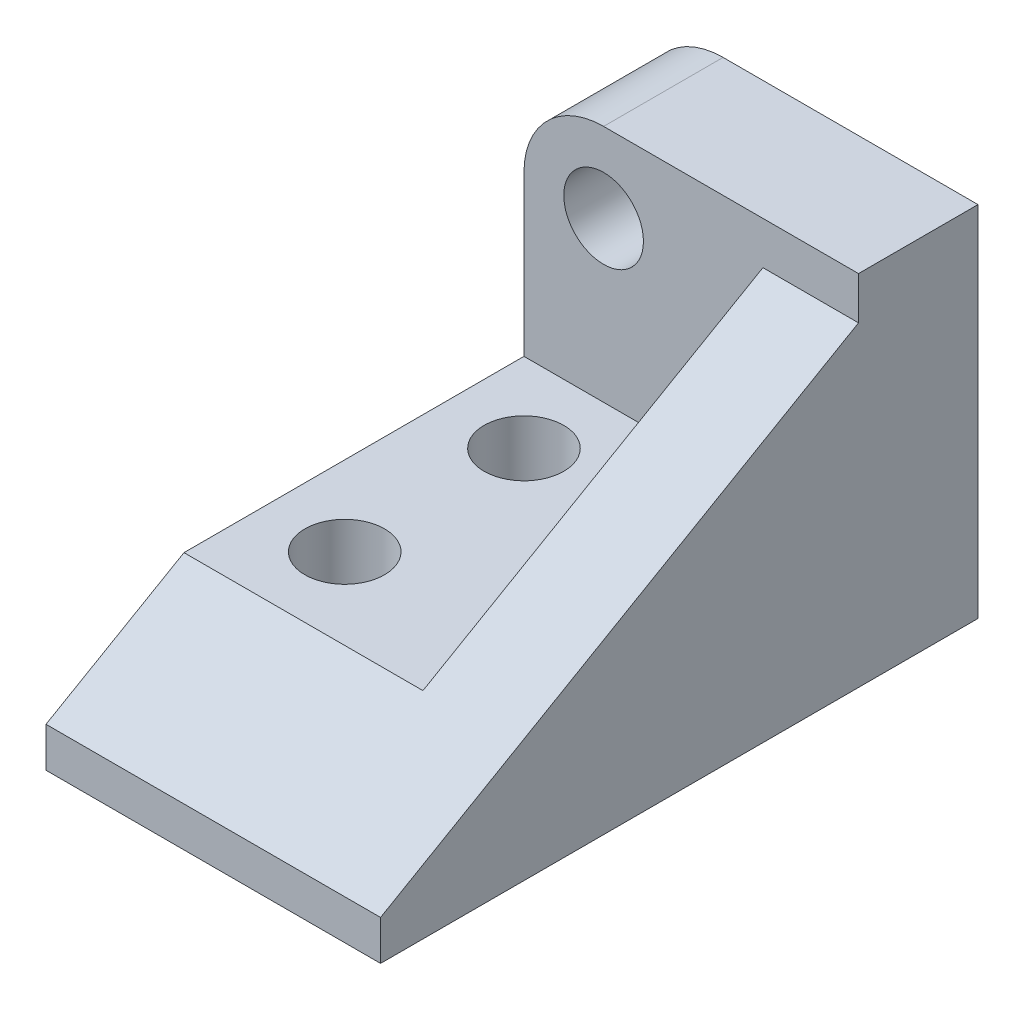
ISO-10303-21;
HEADER;
FILE_DESCRIPTION(('STEP AP214'),'2;1');
FILE_NAME('part.step','',(''),(''),'','','');
FILE_SCHEMA(('AUTOMOTIVE_DESIGN { 1 0 10303 214 1 1 1 1 }'));
ENDSEC;
DATA;
#1=APPLICATION_CONTEXT('core data for automotive mechanical design processes');
#2=APPLICATION_PROTOCOL_DEFINITION('international standard','automotive_design',2000,#1);
#3=PRODUCT_CONTEXT('',#1,'mechanical');
#4=PRODUCT('Part','Part','',(#3));
#5=PRODUCT_RELATED_PRODUCT_CATEGORY('part','',(#4));
#6=PRODUCT_DEFINITION_FORMATION('','',#4);
#7=PRODUCT_DEFINITION_CONTEXT('part definition',#1,'design');
#8=PRODUCT_DEFINITION('design','',#6,#7);
#9=PRODUCT_DEFINITION_SHAPE('','',#8);
#10=(LENGTH_UNIT() NAMED_UNIT(*) SI_UNIT(.MILLI.,.METRE.));
#11=(NAMED_UNIT(*) PLANE_ANGLE_UNIT() SI_UNIT($,.RADIAN.));
#12=(NAMED_UNIT(*) SI_UNIT($,.STERADIAN.) SOLID_ANGLE_UNIT());
#13=UNCERTAINTY_MEASURE_WITH_UNIT(LENGTH_MEASURE(1.E-05),#10,'distance_accuracy_value','');
#14=(GEOMETRIC_REPRESENTATION_CONTEXT(3) GLOBAL_UNCERTAINTY_ASSIGNED_CONTEXT((#13)) GLOBAL_UNIT_ASSIGNED_CONTEXT((#10,
#11,#12)) REPRESENTATION_CONTEXT('',''));
#15=CARTESIAN_POINT('',(0.,0.,0.));
#16=DIRECTION('',(0.,0.,1.));
#17=DIRECTION('',(1.,0.,0.));
#18=AXIS2_PLACEMENT_3D('',#15,#16,#17);
#19=CARTESIAN_POINT('',(-84.,30.,0.));
#20=DIRECTION('',(0.,1.,0.));
#21=DIRECTION('',(0.,0.,1.));
#22=AXIS2_PLACEMENT_3D('',#19,#20,#21);
#23=PLANE('',#22);
#24=CARTESIAN_POINT('',(-64.,30.,-100.));
#25=DIRECTION('',(0.,1.,0.));
#26=DIRECTION('',(0.,0.,1.));
#27=AXIS2_PLACEMENT_3D('',#24,#25,#26);
#28=CIRCLE('',#27,10.);
#29=CARTESIAN_POINT('',(-64.,30.,-90.));
#30=VERTEX_POINT('',#29);
#31=EDGE_CURVE('E126',#30,#30,#28,.T.);
#32=ORIENTED_EDGE('',*,*,#31,.F.);
#33=EDGE_LOOP('',(#32));
#34=FACE_BOUND('',#33,.T.);
#35=CARTESIAN_POINT('',(-64.,30.,-55.));
#36=DIRECTION('',(0.,1.,0.));
#37=DIRECTION('',(0.,0.,1.));
#38=AXIS2_PLACEMENT_3D('',#35,#36,#37);
#39=CIRCLE('',#38,10.);
#40=CARTESIAN_POINT('',(-64.,30.,-45.));
#41=VERTEX_POINT('',#40);
#42=EDGE_CURVE('E268',#41,#41,#39,.T.);
#43=ORIENTED_EDGE('',*,*,#42,.F.);
#44=EDGE_LOOP('',(#43));
#45=FACE_BOUND('',#44,.T.);
#46=DIRECTION('',(1.,0.,0.));
#47=VECTOR('',#46,1.);
#48=CARTESIAN_POINT('',(-84.,30.,-34.6410161513771));
#49=LINE('',#48,#47);
#50=CARTESIAN_POINT('',(-84.,30.,-34.6410161513771));
#51=VERTEX_POINT('',#50);
#52=CARTESIAN_POINT('',(-24.,30.,-34.6410161513771));
#53=VERTEX_POINT('',#52);
#54=EDGE_CURVE('E129',#51,#53,#49,.T.);
#55=ORIENTED_EDGE('',*,*,#54,.T.);
#56=DIRECTION('',(0.,0.,-1.));
#57=VECTOR('',#56,1.);
#58=CARTESIAN_POINT('',(-24.,30.,-120.));
#59=LINE('',#58,#57);
#60=CARTESIAN_POINT('',(-24.,30.,-120.));
#61=VERTEX_POINT('',#60);
#62=EDGE_CURVE('E116',#53,#61,#59,.T.);
#63=ORIENTED_EDGE('',*,*,#62,.T.);
#64=DIRECTION('',(1.,0.,0.));
#65=VECTOR('',#64,1.);
#66=CARTESIAN_POINT('',(-84.,30.,-120.));
#67=LINE('',#66,#65);
#68=CARTESIAN_POINT('',(-84.,30.,-120.));
#69=VERTEX_POINT('',#68);
#70=EDGE_CURVE('E127',#69,#61,#67,.T.);
#71=ORIENTED_EDGE('',*,*,#70,.F.);
#72=DIRECTION('',(0.,0.,1.));
#73=VECTOR('',#72,1.);
#74=CARTESIAN_POINT('',(-84.,30.,0.));
#75=LINE('',#74,#73);
#76=EDGE_CURVE('E191',#69,#51,#75,.T.);
#77=ORIENTED_EDGE('',*,*,#76,.T.);
#78=EDGE_LOOP('',(#55,#63,#71,#77));
#79=FACE_BOUND('',#78,.T.);
#80=ADVANCED_FACE('F43',(#34,#45,#79),#23,.T.);
#81=CARTESIAN_POINT('',(-84.,0.,-120.));
#82=DIRECTION('',(0.,0.,1.));
#83=DIRECTION('',(1.,0.,0.));
#84=AXIS2_PLACEMENT_3D('',#81,#82,#83);
#85=PLANE('',#84);
#86=CARTESIAN_POINT('',(-64.,70.,-120.));
#87=DIRECTION('',(0.,0.,1.));
#88=DIRECTION('',(1.,0.,0.));
#89=AXIS2_PLACEMENT_3D('',#86,#87,#88);
#90=CIRCLE('',#89,10.);
#91=CARTESIAN_POINT('',(-54.,70.,-120.));
#92=VERTEX_POINT('',#91);
#93=EDGE_CURVE('E144',#92,#92,#90,.T.);
#94=ORIENTED_EDGE('',*,*,#93,.F.);
#95=EDGE_LOOP('',(#94));
#96=FACE_BOUND('',#95,.T.);
#97=DIRECTION('',(1.,0.,0.));
#98=VECTOR('',#97,1.);
#99=CARTESIAN_POINT('',(-84.,90.,-120.));
#100=LINE('',#99,#98);
#101=CARTESIAN_POINT('',(-64.,90.,-120.));
#102=VERTEX_POINT('',#101);
#103=CARTESIAN_POINT('',(0.,90.,-120.));
#104=VERTEX_POINT('',#103);
#105=EDGE_CURVE('E149',#102,#104,#100,.T.);
#106=ORIENTED_EDGE('',*,*,#105,.F.);
#107=CARTESIAN_POINT('',(-64.,70.,-120.));
#108=DIRECTION('',(0.,0.,1.));
#109=DIRECTION('',(1.,0.,0.));
#110=AXIS2_PLACEMENT_3D('',#107,#108,#109);
#111=CIRCLE('',#110,20.);
#112=CARTESIAN_POINT('',(-84.,70.,-120.));
#113=VERTEX_POINT('',#112);
#114=EDGE_CURVE('E63',#102,#113,#111,.T.);
#115=ORIENTED_EDGE('',*,*,#114,.T.);
#116=DIRECTION('',(0.,-1.,0.));
#117=VECTOR('',#116,1.);
#118=CARTESIAN_POINT('',(-84.,0.,-120.));
#119=LINE('',#118,#117);
#120=EDGE_CURVE('E131',#113,#69,#119,.T.);
#121=ORIENTED_EDGE('',*,*,#120,.T.);
#122=ORIENTED_EDGE('',*,*,#70,.T.);
#123=DIRECTION('',(0.,1.,0.));
#124=VECTOR('',#123,1.);
#125=CARTESIAN_POINT('',(-24.,79.2820323027558,-120.));
#126=LINE('',#125,#124);
#127=CARTESIAN_POINT('',(-24.,79.2820323027558,-120.));
#128=VERTEX_POINT('',#127);
#129=EDGE_CURVE('E113',#61,#128,#126,.T.);
#130=ORIENTED_EDGE('',*,*,#129,.T.);
#131=DIRECTION('',(1.,0.,0.));
#132=VECTOR('',#131,1.);
#133=CARTESIAN_POINT('',(-24.,79.2820323027558,-120.));
#134=LINE('',#133,#132);
#135=CARTESIAN_POINT('',(0.,79.2820323027558,-120.));
#136=VERTEX_POINT('',#135);
#137=EDGE_CURVE('E189',#128,#136,#134,.T.);
#138=ORIENTED_EDGE('',*,*,#137,.T.);
#139=DIRECTION('',(0.,-1.,0.));
#140=VECTOR('',#139,1.);
#141=CARTESIAN_POINT('',(0.,0.,-120.));
#142=LINE('',#141,#140);
#143=EDGE_CURVE('E187',#104,#136,#142,.T.);
#144=ORIENTED_EDGE('',*,*,#143,.F.);
#145=EDGE_LOOP('',(#106,#115,#121,#122,#130,#138,#144));
#146=FACE_BOUND('',#145,.T.);
#147=ADVANCED_FACE('F134',(#96,#146),#85,.T.);
#148=CARTESIAN_POINT('',(-84.,90.,0.));
#149=DIRECTION('',(0.,1.,0.));
#150=DIRECTION('',(0.,0.,1.));
#151=AXIS2_PLACEMENT_3D('',#148,#149,#150);
#152=PLANE('',#151);
#153=DIRECTION('',(1.,0.,0.));
#154=VECTOR('',#153,1.);
#155=CARTESIAN_POINT('',(-84.,90.,-150.));
#156=LINE('',#155,#154);
#157=CARTESIAN_POINT('',(-64.,90.,-150.));
#158=VERTEX_POINT('',#157);
#159=CARTESIAN_POINT('',(0.,90.,-150.));
#160=VERTEX_POINT('',#159);
#161=EDGE_CURVE('E151',#158,#160,#156,.T.);
#162=ORIENTED_EDGE('',*,*,#161,.F.);
#163=DIRECTION('',(0.,0.,1.));
#164=VECTOR('',#163,1.);
#165=CARTESIAN_POINT('',(-64.,90.,-120.));
#166=LINE('',#165,#164);
#167=EDGE_CURVE('E143',#158,#102,#166,.T.);
#168=ORIENTED_EDGE('',*,*,#167,.T.);
#169=ORIENTED_EDGE('',*,*,#105,.T.);
#170=DIRECTION('',(0.,0.,1.));
#171=VECTOR('',#170,1.);
#172=CARTESIAN_POINT('',(0.,90.,0.));
#173=LINE('',#172,#171);
#174=EDGE_CURVE('E159',#160,#104,#173,.T.);
#175=ORIENTED_EDGE('',*,*,#174,.F.);
#176=EDGE_LOOP('',(#162,#168,#169,#175));
#177=FACE_BOUND('',#176,.T.);
#178=ADVANCED_FACE('F230',(#177),#152,.T.);
#179=CARTESIAN_POINT('',(-84.,0.,-150.));
#180=DIRECTION('',(0.,0.,-1.));
#181=DIRECTION('',(-1.,0.,0.));
#182=AXIS2_PLACEMENT_3D('',#179,#180,#181);
#183=PLANE('',#182);
#184=CARTESIAN_POINT('',(-64.,70.,-150.));
#185=DIRECTION('',(0.,0.,-1.));
#186=DIRECTION('',(-1.,0.,0.));
#187=AXIS2_PLACEMENT_3D('',#184,#185,#186);
#188=CIRCLE('',#187,10.);
#189=CARTESIAN_POINT('',(-54.,70.,-150.));
#190=VERTEX_POINT('',#189);
#191=EDGE_CURVE('E142',#190,#190,#188,.T.);
#192=ORIENTED_EDGE('',*,*,#191,.F.);
#193=EDGE_LOOP('',(#192));
#194=FACE_BOUND('',#193,.T.);
#195=DIRECTION('',(0.,1.,0.));
#196=VECTOR('',#195,1.);
#197=CARTESIAN_POINT('',(-84.,0.,-150.));
#198=LINE('',#197,#196);
#199=CARTESIAN_POINT('',(-84.,0.,-150.));
#200=VERTEX_POINT('',#199);
#201=CARTESIAN_POINT('',(-84.,70.,-150.));
#202=VERTEX_POINT('',#201);
#203=EDGE_CURVE('E135',#200,#202,#198,.T.);
#204=ORIENTED_EDGE('',*,*,#203,.T.);
#205=CARTESIAN_POINT('',(-64.,70.,-150.));
#206=DIRECTION('',(0.,0.,-1.));
#207=DIRECTION('',(-1.,0.,0.));
#208=AXIS2_PLACEMENT_3D('',#205,#206,#207);
#209=CIRCLE('',#208,20.);
#210=EDGE_CURVE('E11',#202,#158,#209,.T.);
#211=ORIENTED_EDGE('',*,*,#210,.T.);
#212=ORIENTED_EDGE('',*,*,#161,.T.);
#213=DIRECTION('',(0.,1.,0.));
#214=VECTOR('',#213,1.);
#215=CARTESIAN_POINT('',(0.,0.,-150.));
#216=LINE('',#215,#214);
#217=CARTESIAN_POINT('',(0.,0.,-150.));
#218=VERTEX_POINT('',#217);
#219=EDGE_CURVE('E192',#218,#160,#216,.T.);
#220=ORIENTED_EDGE('',*,*,#219,.F.);
#221=DIRECTION('',(1.,0.,0.));
#222=VECTOR('',#221,1.);
#223=CARTESIAN_POINT('',(-84.,0.,-150.));
#224=LINE('',#223,#222);
#225=EDGE_CURVE('E158',#200,#218,#224,.T.);
#226=ORIENTED_EDGE('',*,*,#225,.F.);
#227=EDGE_LOOP('',(#204,#211,#212,#220,#226));
#228=FACE_BOUND('',#227,.T.);
#229=ADVANCED_FACE('F208',(#194,#228),#183,.T.);
#230=CARTESIAN_POINT('',(-84.,0.,0.));
#231=DIRECTION('',(0.,-1.,0.));
#232=DIRECTION('',(0.,0.,-1.));
#233=AXIS2_PLACEMENT_3D('',#230,#231,#232);
#234=PLANE('',#233);
#235=CARTESIAN_POINT('',(-64.,0.,-100.));
#236=DIRECTION('',(0.,1.,0.));
#237=DIRECTION('',(0.,0.,1.));
#238=AXIS2_PLACEMENT_3D('',#235,#236,#237);
#239=CIRCLE('',#238,10.);
#240=CARTESIAN_POINT('',(-64.,0.,-90.));
#241=VERTEX_POINT('',#240);
#242=EDGE_CURVE('E264',#241,#241,#239,.T.);
#243=ORIENTED_EDGE('',*,*,#242,.T.);
#244=EDGE_LOOP('',(#243));
#245=FACE_BOUND('',#244,.T.);
#246=CARTESIAN_POINT('',(-64.,0.,-55.));
#247=DIRECTION('',(0.,1.,0.));
#248=DIRECTION('',(0.,0.,1.));
#249=AXIS2_PLACEMENT_3D('',#246,#247,#248);
#250=CIRCLE('',#249,10.);
#251=CARTESIAN_POINT('',(-64.,0.,-45.));
#252=VERTEX_POINT('',#251);
#253=EDGE_CURVE('E261',#252,#252,#250,.T.);
#254=ORIENTED_EDGE('',*,*,#253,.T.);
#255=EDGE_LOOP('',(#254));
#256=FACE_BOUND('',#255,.T.);
#257=DIRECTION('',(0.,0.,-1.));
#258=VECTOR('',#257,1.);
#259=CARTESIAN_POINT('',(0.,0.,0.));
#260=LINE('',#259,#258);
#261=CARTESIAN_POINT('',(0.,0.,0.));
#262=VERTEX_POINT('',#261);
#263=EDGE_CURVE('E181',#262,#218,#260,.T.);
#264=ORIENTED_EDGE('',*,*,#263,.F.);
#265=DIRECTION('',(1.,0.,0.));
#266=VECTOR('',#265,1.);
#267=CARTESIAN_POINT('',(-84.,0.,0.));
#268=LINE('',#267,#266);
#269=CARTESIAN_POINT('',(-84.,0.,0.));
#270=VERTEX_POINT('',#269);
#271=EDGE_CURVE('E161',#270,#262,#268,.T.);
#272=ORIENTED_EDGE('',*,*,#271,.F.);
#273=DIRECTION('',(0.,0.,-1.));
#274=VECTOR('',#273,1.);
#275=CARTESIAN_POINT('',(-84.,0.,0.));
#276=LINE('',#275,#274);
#277=EDGE_CURVE('E140',#270,#200,#276,.T.);
#278=ORIENTED_EDGE('',*,*,#277,.T.);
#279=ORIENTED_EDGE('',*,*,#225,.T.);
#280=EDGE_LOOP('',(#264,#272,#278,#279));
#281=FACE_BOUND('',#280,.T.);
#282=ADVANCED_FACE('F207',(#245,#256,#281),#234,.T.);
#283=CARTESIAN_POINT('',(-84.,0.,0.));
#284=DIRECTION('',(0.,0.,-1.));
#285=DIRECTION('',(-1.,0.,0.));
#286=AXIS2_PLACEMENT_3D('',#283,#284,#285);
#287=PLANE('',#286);
#288=DIRECTION('',(0.,1.,0.));
#289=VECTOR('',#288,1.);
#290=CARTESIAN_POINT('',(0.,0.,0.));
#291=LINE('',#290,#289);
#292=CARTESIAN_POINT('',(0.,10.,0.));
#293=VERTEX_POINT('',#292);
#294=EDGE_CURVE('E176',#262,#293,#291,.T.);
#295=ORIENTED_EDGE('',*,*,#294,.T.);
#296=DIRECTION('',(1.,0.,0.));
#297=VECTOR('',#296,1.);
#298=CARTESIAN_POINT('',(-84.,10.,0.));
#299=LINE('',#298,#297);
#300=CARTESIAN_POINT('',(-84.,10.,0.));
#301=VERTEX_POINT('',#300);
#302=EDGE_CURVE('E132',#301,#293,#299,.T.);
#303=ORIENTED_EDGE('',*,*,#302,.F.);
#304=DIRECTION('',(0.,1.,0.));
#305=VECTOR('',#304,1.);
#306=CARTESIAN_POINT('',(-84.,0.,0.));
#307=LINE('',#306,#305);
#308=EDGE_CURVE('E203',#270,#301,#307,.T.);
#309=ORIENTED_EDGE('',*,*,#308,.F.);
#310=ORIENTED_EDGE('',*,*,#271,.T.);
#311=EDGE_LOOP('',(#295,#303,#309,#310));
#312=FACE_BOUND('',#311,.T.);
#313=ADVANCED_FACE('F180',(#312),#287,.F.);
#314=CARTESIAN_POINT('',(-84.,7.49999999999995,4.33012701892221));
#315=DIRECTION('',(0.,0.866025403784436,0.500000000000004));
#316=DIRECTION('',(0.,-0.500000000000004,0.866025403784436));
#317=AXIS2_PLACEMENT_3D('',#314,#315,#316);
#318=PLANE('',#317);
#319=DIRECTION('',(0.,-0.500000000000004,0.866025403784436));
#320=VECTOR('',#319,1.);
#321=CARTESIAN_POINT('',(0.,7.49999999999995,4.33012701892221));
#322=LINE('',#321,#320);
#323=EDGE_CURVE('E167',#136,#293,#322,.T.);
#324=ORIENTED_EDGE('',*,*,#323,.F.);
#325=ORIENTED_EDGE('',*,*,#137,.F.);
#326=DIRECTION('',(0.,-0.500000000000004,0.866025403784436));
#327=VECTOR('',#326,1.);
#328=CARTESIAN_POINT('',(-24.,30.,-34.6410161513771));
#329=LINE('',#328,#327);
#330=EDGE_CURVE('E117',#128,#53,#329,.T.);
#331=ORIENTED_EDGE('',*,*,#330,.T.);
#332=ORIENTED_EDGE('',*,*,#54,.F.);
#333=DIRECTION('',(0.,-0.500000000000004,0.866025403784436));
#334=VECTOR('',#333,1.);
#335=CARTESIAN_POINT('',(-84.,7.49999999999995,4.33012701892221));
#336=LINE('',#335,#334);
#337=EDGE_CURVE('E175',#51,#301,#336,.T.);
#338=ORIENTED_EDGE('',*,*,#337,.T.);
#339=ORIENTED_EDGE('',*,*,#302,.T.);
#340=EDGE_LOOP('',(#324,#325,#331,#332,#338,#339));
#341=FACE_BOUND('',#340,.T.);
#342=ADVANCED_FACE('F166',(#341),#318,.T.);
#343=CARTESIAN_POINT('',(-84.,0.,0.));
#344=DIRECTION('',(1.,0.,0.));
#345=DIRECTION('',(0.,0.,-1.));
#346=AXIS2_PLACEMENT_3D('',#343,#344,#345);
#347=PLANE('',#346);
#348=ORIENTED_EDGE('',*,*,#120,.F.);
#349=DIRECTION('',(0.,0.,1.));
#350=VECTOR('',#349,1.);
#351=CARTESIAN_POINT('',(-84.,70.,-150.));
#352=LINE('',#351,#350);
#353=EDGE_CURVE('E51',#113,#202,#352,.F.);
#354=ORIENTED_EDGE('',*,*,#353,.T.);
#355=ORIENTED_EDGE('',*,*,#203,.F.);
#356=ORIENTED_EDGE('',*,*,#277,.F.);
#357=ORIENTED_EDGE('',*,*,#308,.T.);
#358=ORIENTED_EDGE('',*,*,#337,.F.);
#359=ORIENTED_EDGE('',*,*,#76,.F.);
#360=EDGE_LOOP('',(#348,#354,#355,#356,#357,#358,#359));
#361=FACE_BOUND('',#360,.T.);
#362=ADVANCED_FACE('F210',(#361),#347,.F.);
#363=CARTESIAN_POINT('',(0.,0.,0.));
#364=DIRECTION('',(1.,0.,0.));
#365=DIRECTION('',(0.,0.,-1.));
#366=AXIS2_PLACEMENT_3D('',#363,#364,#365);
#367=PLANE('',#366);
#368=ORIENTED_EDGE('',*,*,#143,.T.);
#369=ORIENTED_EDGE('',*,*,#323,.T.);
#370=ORIENTED_EDGE('',*,*,#294,.F.);
#371=ORIENTED_EDGE('',*,*,#263,.T.);
#372=ORIENTED_EDGE('',*,*,#219,.T.);
#373=ORIENTED_EDGE('',*,*,#174,.T.);
#374=EDGE_LOOP('',(#368,#369,#370,#371,#372,#373));
#375=FACE_BOUND('',#374,.T.);
#376=ADVANCED_FACE('F183',(#375),#367,.T.);
#377=CARTESIAN_POINT('',(-24.,0.,0.));
#378=DIRECTION('',(1.,0.,0.));
#379=DIRECTION('',(0.,0.,-1.));
#380=AXIS2_PLACEMENT_3D('',#377,#378,#379);
#381=PLANE('',#380);
#382=ORIENTED_EDGE('',*,*,#62,.F.);
#383=ORIENTED_EDGE('',*,*,#330,.F.);
#384=ORIENTED_EDGE('',*,*,#129,.F.);
#385=EDGE_LOOP('',(#382,#383,#384));
#386=FACE_BOUND('',#385,.T.);
#387=ADVANCED_FACE('F114',(#386),#381,.F.);
#388=CARTESIAN_POINT('',(-64.,30.,-55.));
#389=DIRECTION('',(0.,-1.,0.));
#390=DIRECTION('',(0.,0.,-1.));
#391=AXIS2_PLACEMENT_3D('',#388,#389,#390);
#392=CYLINDRICAL_SURFACE('',#391,10.);
#393=ORIENTED_EDGE('',*,*,#42,.T.);
#394=EDGE_LOOP('',(#393));
#395=FACE_BOUND('',#394,.T.);
#396=ORIENTED_EDGE('',*,*,#253,.F.);
#397=EDGE_LOOP('',(#396));
#398=FACE_BOUND('',#397,.T.);
#399=ADVANCED_FACE('F248',(#395,#398),#392,.F.);
#400=CARTESIAN_POINT('',(-64.,30.,-100.));
#401=DIRECTION('',(0.,-1.,0.));
#402=DIRECTION('',(0.,0.,-1.));
#403=AXIS2_PLACEMENT_3D('',#400,#401,#402);
#404=CYLINDRICAL_SURFACE('',#403,10.);
#405=ORIENTED_EDGE('',*,*,#31,.T.);
#406=EDGE_LOOP('',(#405));
#407=FACE_BOUND('',#406,.T.);
#408=ORIENTED_EDGE('',*,*,#242,.F.);
#409=EDGE_LOOP('',(#408));
#410=FACE_BOUND('',#409,.T.);
#411=ADVANCED_FACE('F220',(#407,#410),#404,.F.);
#412=CARTESIAN_POINT('',(-64.,70.,-208.));
#413=DIRECTION('',(0.,0.,1.));
#414=DIRECTION('',(1.,0.,0.));
#415=AXIS2_PLACEMENT_3D('',#412,#413,#414);
#416=CYLINDRICAL_SURFACE('',#415,10.);
#417=CARTESIAN_POINT('',(-54.,70.,-120.));
#418=CARTESIAN_POINT('',(-54.,70.,-120.3125));
#419=CARTESIAN_POINT('',(-54.,70.,-120.625));
#420=CARTESIAN_POINT('',(-54.,70.,-121.25));
#421=CARTESIAN_POINT('',(-54.,70.,-121.5625));
#422=CARTESIAN_POINT('',(-54.,70.,-122.1875));
#423=CARTESIAN_POINT('',(-54.,70.,-122.5));
#424=CARTESIAN_POINT('',(-54.,70.,-123.125));
#425=CARTESIAN_POINT('',(-54.,70.,-123.4375));
#426=CARTESIAN_POINT('',(-54.,70.,-124.0625));
#427=CARTESIAN_POINT('',(-54.,70.,-124.375));
#428=CARTESIAN_POINT('',(-54.,70.,-125.));
#429=CARTESIAN_POINT('',(-54.,70.,-125.3125));
#430=CARTESIAN_POINT('',(-54.,70.,-125.9375));
#431=CARTESIAN_POINT('',(-54.,70.,-126.25));
#432=CARTESIAN_POINT('',(-54.,70.,-126.875));
#433=CARTESIAN_POINT('',(-54.,70.,-127.1875));
#434=CARTESIAN_POINT('',(-54.,70.,-127.8125));
#435=CARTESIAN_POINT('',(-54.,70.,-128.125));
#436=CARTESIAN_POINT('',(-54.,70.,-128.75));
#437=CARTESIAN_POINT('',(-54.,70.,-129.0625));
#438=CARTESIAN_POINT('',(-54.,70.,-129.6875));
#439=CARTESIAN_POINT('',(-54.,70.,-130.));
#440=CARTESIAN_POINT('',(-54.,70.,-130.625));
#441=CARTESIAN_POINT('',(-54.,70.,-130.9375));
#442=CARTESIAN_POINT('',(-54.,70.,-131.5625));
#443=CARTESIAN_POINT('',(-54.,70.,-131.875));
#444=CARTESIAN_POINT('',(-54.,70.,-132.5));
#445=CARTESIAN_POINT('',(-54.,70.,-132.8125));
#446=CARTESIAN_POINT('',(-54.,70.,-133.4375));
#447=CARTESIAN_POINT('',(-54.,70.,-133.75));
#448=CARTESIAN_POINT('',(-54.,70.,-134.375));
#449=CARTESIAN_POINT('',(-54.,70.,-134.6875));
#450=CARTESIAN_POINT('',(-54.,70.,-135.3125));
#451=CARTESIAN_POINT('',(-54.,70.,-135.625));
#452=CARTESIAN_POINT('',(-54.,70.,-136.25));
#453=CARTESIAN_POINT('',(-54.,70.,-136.5625));
#454=CARTESIAN_POINT('',(-54.,70.,-137.1875));
#455=CARTESIAN_POINT('',(-54.,70.,-137.5));
#456=CARTESIAN_POINT('',(-54.,70.,-138.125));
#457=CARTESIAN_POINT('',(-54.,70.,-138.4375));
#458=CARTESIAN_POINT('',(-54.,70.,-139.0625));
#459=CARTESIAN_POINT('',(-54.,70.,-139.375));
#460=CARTESIAN_POINT('',(-54.,70.,-140.));
#461=CARTESIAN_POINT('',(-54.,70.,-140.3125));
#462=CARTESIAN_POINT('',(-54.,70.,-140.9375));
#463=CARTESIAN_POINT('',(-54.,70.,-141.25));
#464=CARTESIAN_POINT('',(-54.,70.,-141.875));
#465=CARTESIAN_POINT('',(-54.,70.,-142.1875));
#466=CARTESIAN_POINT('',(-54.,70.,-142.8125));
#467=CARTESIAN_POINT('',(-54.,70.,-143.125));
#468=CARTESIAN_POINT('',(-54.,70.,-143.75));
#469=CARTESIAN_POINT('',(-54.,70.,-144.0625));
#470=CARTESIAN_POINT('',(-54.,70.,-144.6875));
#471=CARTESIAN_POINT('',(-54.,70.,-145.));
#472=CARTESIAN_POINT('',(-54.,70.,-145.625));
#473=CARTESIAN_POINT('',(-54.,70.,-145.9375));
#474=CARTESIAN_POINT('',(-54.,70.,-146.5625));
#475=CARTESIAN_POINT('',(-54.,70.,-146.875));
#476=CARTESIAN_POINT('',(-54.,70.,-147.5));
#477=CARTESIAN_POINT('',(-54.,70.,-147.8125));
#478=CARTESIAN_POINT('',(-54.,70.,-148.4375));
#479=CARTESIAN_POINT('',(-54.,70.,-148.75));
#480=CARTESIAN_POINT('',(-54.,70.,-149.375));
#481=CARTESIAN_POINT('',(-54.,70.,-149.6875));
#482=CARTESIAN_POINT('',(-54.,70.,-150.));
#483=B_SPLINE_CURVE_WITH_KNOTS('',3,(#417,#418,#419,#420,#421,#422,#423,#424,#425,#426,#427,
#428,#429,#430,#431,#432,#433,#434,#435,#436,#437,#438,#439,#440,#441,#442,#443,#444,#445,#446,
#447,#448,#449,#450,#451,#452,#453,#454,#455,#456,#457,#458,#459,#460,#461,#462,#463,#464,#465,
#466,#467,#468,#469,#470,#471,#472,#473,#474,#475,#476,#477,#478,#479,#480,#481,#482),
.UNSPECIFIED.,.F.,.F.,(4,2,2,2,2,2,2,2,2,2,2,2,2,2,2,2,2,2,2,2,2,2,2,2,2,2,2,2,2,2,2,2,4),(0.,
0.937499999999994,1.875,2.8125,3.75,4.6875,5.62499999999999,6.5625,7.50000000000001,
8.43749999999999,9.37499999999999,10.3125,11.25,12.1875,13.125,14.0625,15.,15.9375,16.875,
17.8125,18.75,19.6875,20.625,21.5625,22.5,23.4375,24.375,25.3125,26.25,27.1875,28.125,29.0625,
30.),.UNSPECIFIED.);
#484=EDGE_CURVE('BSEAM214',#92,#190,#483,.T.);
#485=ORIENTED_EDGE('',*,*,#93,.T.);
#486=ORIENTED_EDGE('',*,*,#191,.T.);
#487=ORIENTED_EDGE('',*,*,#484,.T.);
#488=ORIENTED_EDGE('',*,*,#484,.F.);
#489=EDGE_LOOP('',(#485,#487,#486,#488));
#490=FACE_BOUND('',#489,.T.);
#491=ADVANCED_FACE('F214',(#490),#416,.F.);
#492=CARTESIAN_POINT('',(-64.,70.,0.));
#493=DIRECTION('',(0.,0.,-1.));
#494=DIRECTION('',(-1.,0.,0.));
#495=AXIS2_PLACEMENT_3D('',#492,#493,#494);
#496=CYLINDRICAL_SURFACE('',#495,20.);
#497=ORIENTED_EDGE('',*,*,#210,.F.);
#498=ORIENTED_EDGE('',*,*,#353,.F.);
#499=ORIENTED_EDGE('',*,*,#114,.F.);
#500=ORIENTED_EDGE('',*,*,#167,.F.);
#501=EDGE_LOOP('',(#497,#498,#499,#500));
#502=FACE_BOUND('',#501,.T.);
#503=ADVANCED_FACE('F44',(#502),#496,.T.);
#504=CLOSED_SHELL('',(#80,#147,#178,#229,#282,#313,#342,#362,#376,#387,#399,#411,#491,#503));
#505=MANIFOLD_SOLID_BREP('B2',#504);
#506=ADVANCED_BREP_SHAPE_REPRESENTATION('',(#18,#505),#14);
#507=SHAPE_DEFINITION_REPRESENTATION(#9,#506);
ENDSEC;
END-ISO-10303-21;
